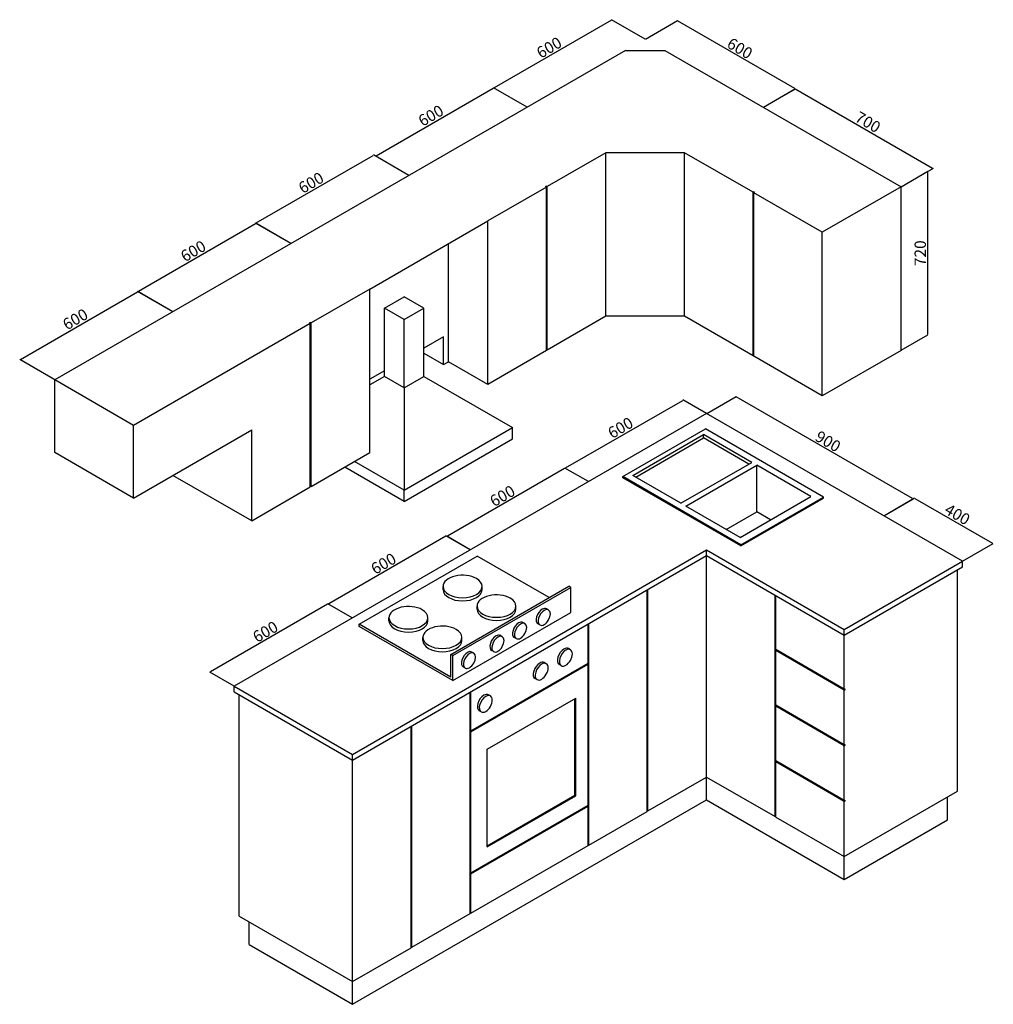
# Model space of a CAD drawing. Units: millimetres. Extents: x 2103 to 6389, y -1168 to 3165.
import ezdxf

# ---------------------------------------------------------------- set-up
doc = ezdxf.new("R2010")
doc.units = ezdxf.units.MM
doc.layers.add('A-ANNO-DIMS', color=2, linetype='Continuous', lineweight=18)
doc.layers.add('A-FURN', color=7, linetype='Continuous', lineweight=25)
doc.styles.get("Standard").update_dxf_attribs({"font": 'arial.ttf'})
doc.dimstyles.new('ISO-25', dxfattribs={"dimtxt": 50, "dimasz": 2.5, "dimexe": 1.25, "dimexo": 0.625, "dimtad": 1, "dimdec": 0, "dimtxsty": 'Standard', "dimcen": 2.5, "dimadec": 0, "dimazin": 0, "dimtfac": 1, "dimtdec": 0, "dimtmove": 0, "dimatfit": 3, "dimfxl": 1, "dimarcsym": 0})

# ---------------------------------------------------------------- blocks, each defined once
blk = doc.blocks.new('*D1')
at = {"layer": 'A-ANNO-DIMS', "color": 0, "lineweight": -2, "transparency": 16777216}
for p, q in [((2106.7, 1670), (2622, 1967.5)), ((2777.4, 1880.3), (2622.9, 1969.5)), ((2257.8, 1580.3), (2103.3, 1669.5))]:
    blk.add_line(p, q, dxfattribs=at)
at = {"layer": 'A-ANNO-DIMS', "color": 0, "transparency": 16777216}
for points in [[(2621.8, 1967.9), (2622.2, 1967.2), (2624.2, 1968.8)], [(2106.5, 1670.4), (2106.9, 1669.7), (2104.6, 1668.8)]]:
    blk.add_solid(points, dxfattribs=at)
at = {"layer": 'Defpoints', "color": 0, "transparency": 16777216}
for p in [(2624.2, 1968.8), (2778, 1879.9), (2258.4, 1579.9)]:
    blk.add_point(p, dxfattribs=at)
at = {"layer": 'A-ANNO-DIMS', "color": 0, "transparency": 16777216, "insert": (2351.3, 1841.4), "char_height": 50, "attachment_point": 5, "rotation": 30}
blk.add_mtext('600', dxfattribs=at)
blk = doc.blocks.new('*D2')
at = {"layer": 'A-ANNO-DIMS', "color": 0, "lineweight": -2, "transparency": 16777216}
for p, q in [((2626, 1970.2), (3141.2, 2267.7)), ((3297, 2180.3), (3142.2, 2269.7)), ((2777.4, 1880.3), (2622.5, 1969.7))]:
    blk.add_line(p, q, dxfattribs=at)
at = {"layer": 'A-ANNO-DIMS', "color": 0, "transparency": 16777216}
for points in [[(3141, 2268.1), (3141.5, 2267.4), (3143.4, 2269)], [(2625.8, 1970.6), (2626.2, 1969.9), (2623.8, 1969)]]:
    blk.add_solid(points, dxfattribs=at)
at = {"layer": 'Defpoints', "color": 0, "transparency": 16777216}
for p in [(3143.4, 2269), (3297.7, 2179.9), (2778, 1879.9)]:
    blk.add_point(p, dxfattribs=at)
at = {"layer": 'A-ANNO-DIMS', "color": 0, "transparency": 16777216, "insert": (2870.5, 2141.6), "char_height": 50, "attachment_point": 5, "rotation": 30}
blk.add_mtext('600', dxfattribs=at)
blk = doc.blocks.new('*D3')
at = {"layer": 'A-ANNO-DIMS', "color": 0, "lineweight": -2, "transparency": 16777216}
for p, q in [((3144.5, 2270.9), (3659.8, 2568.4)), ((3816.6, 2480.3), (3660.7, 2570.4)), ((3297, 2180.3), (3141.1, 2270.4))]:
    blk.add_line(p, q, dxfattribs=at)
at = {"layer": 'A-ANNO-DIMS', "color": 0, "transparency": 16777216}
for points in [[(3659.5, 2568.7), (3660, 2568), (3661.9, 2569.6)], [(3144.3, 2271.2), (3144.7, 2270.5), (3142.3, 2269.6)]]:
    blk.add_solid(points, dxfattribs=at)
at = {"layer": 'Defpoints', "color": 0, "transparency": 16777216}
for p in [(3661.9, 2569.6), (3817.3, 2479.9), (3297.7, 2179.9)]:
    blk.add_point(p, dxfattribs=at)
at = {"layer": 'A-ANNO-DIMS', "color": 0, "transparency": 16777216, "insert": (3389, 2442.3), "char_height": 50, "attachment_point": 5, "rotation": 30}
blk.add_mtext('600', dxfattribs=at)
blk = doc.blocks.new('*D4')
at = {"layer": 'A-ANNO-DIMS', "color": 0, "lineweight": -2, "transparency": 16777216}
for p, q in [((3671.8, 2566.4), (4187.1, 2863.9)), ((4336.3, 2780.3), (4188, 2865.9)), ((3816.6, 2480.3), (3668.4, 2565.9))]:
    blk.add_line(p, q, dxfattribs=at)
at = {"layer": 'A-ANNO-DIMS', "color": 0, "transparency": 16777216}
for points in [[(4186.9, 2864.3), (4187.3, 2863.5), (4189.3, 2865.2)], [(3671.6, 2566.8), (3672.1, 2566), (3669.7, 2565.2)]]:
    blk.add_solid(points, dxfattribs=at)
at = {"layer": 'Defpoints', "color": 0, "transparency": 16777216}
for p in [(4189.3, 2865.2), (4336.9, 2779.9), (3817.3, 2479.9)]:
    blk.add_point(p, dxfattribs=at)
at = {"layer": 'A-ANNO-DIMS', "color": 0, "transparency": 16777216, "insert": (3916.4, 2737.8), "char_height": 50, "attachment_point": 5, "rotation": 30}
blk.add_mtext('600', dxfattribs=at)
blk = doc.blocks.new('*D5')
at = {"layer": 'A-ANNO-DIMS', "color": 0, "lineweight": -2, "transparency": 16777216}
for p, q in [((5983, 2430.3), (6100.8, 2498.4)), ((6099.6, 2495.1), (6099.6, 1780.1)), ((5983, 1710.3), (6100.8, 1778.4))]:
    blk.add_line(p, q, dxfattribs=at)
at = {"layer": 'A-ANNO-DIMS', "color": 0, "transparency": 16777216}
for points in [[(6099.2, 2495.1), (6100, 2495.1), (6099.6, 2497.6)], [(6099.2, 1780.1), (6100, 1780.1), (6099.6, 1777.6)]]:
    blk.add_solid(points, dxfattribs=at)
at = {"layer": 'Defpoints', "color": 0, "transparency": 16777216}
for p in [(5982.3, 2429.9), (6099.6, 1777.6), (5982.3, 1709.9)]:
    blk.add_point(p, dxfattribs=at)
at = {"layer": 'A-ANNO-DIMS', "color": 0, "transparency": 16777216, "insert": (6073.4, 2137.6), "char_height": 50, "attachment_point": 5, "rotation": 90}
blk.add_mtext('720', dxfattribs=at)
blk = doc.blocks.new('*D6')
at = {"layer": 'A-ANNO-DIMS', "color": 0, "lineweight": -2, "transparency": 16777216}
for p, q in [((5376.7, 2780.3), (5518.4, 2862.1)), ((5519.3, 2860.1), (6121.2, 2512.6)), ((5983, 2430.3), (6124.6, 2512.1))]:
    blk.add_line(p, q, dxfattribs=at)
at = {"layer": 'A-ANNO-DIMS', "color": 0, "transparency": 16777216}
for points in [[(5519.5, 2860.5), (5519.1, 2859.7), (5517.1, 2861.4)], [(6121.4, 2513), (6121, 2512.2), (6123.3, 2511.4)]]:
    blk.add_solid(points, dxfattribs=at)
at = {"layer": 'Defpoints', "color": 0, "transparency": 16777216}
for p in [(5376.1, 2779.9), (6123.3, 2511.4), (5982.3, 2429.9)]:
    blk.add_point(p, dxfattribs=at)
at = {"layer": 'A-ANNO-DIMS', "color": 0, "transparency": 16777216, "insert": (5833.3, 2709), "char_height": 50, "attachment_point": 5, "rotation": 330}
blk.add_mtext('700', dxfattribs=at)
blk = doc.blocks.new('*D7')
at = {"layer": 'A-ANNO-DIMS', "color": 0, "lineweight": -2, "transparency": 16777216}
for p, q in [((5906.5, 982.2), (6042.1, 1060.5)), ((6043, 1058.6), (6385.1, 861.1)), ((6252.9, 782.2), (6388.5, 860.5))]:
    blk.add_line(p, q, dxfattribs=at)
at = {"layer": 'A-ANNO-DIMS', "color": 0, "transparency": 16777216}
for points in [[(6043.2, 1058.9), (6042.8, 1058.2), (6040.9, 1059.8)], [(6385.3, 861.4), (6384.9, 860.7), (6387.3, 859.8)]]:
    blk.add_solid(points, dxfattribs=at)
at = {"layer": 'Defpoints', "color": 0, "transparency": 16777216}
for p in [(5905.9, 981.9), (6387.3, 859.8), (6252.3, 781.9)]:
    blk.add_point(p, dxfattribs=at)
at = {"layer": 'A-ANNO-DIMS', "color": 0, "transparency": 16777216, "insert": (6227.1, 982.5), "char_height": 50, "attachment_point": 5, "rotation": 330}
blk.add_mtext('400', dxfattribs=at)
blk = doc.blocks.new('*D8')
at = {"layer": 'A-ANNO-DIMS', "color": 0, "lineweight": -2, "transparency": 16777216}
for p, q in [((5127.1, 1432.2), (5256.3, 1506.8)), ((6032.3, 1057.4), (5257.2, 1504.9)), ((5906.5, 982.2), (6035.7, 1056.8))]:
    blk.add_line(p, q, dxfattribs=at)
at = {"layer": 'A-ANNO-DIMS', "color": 0, "transparency": 16777216}
for points in [[(5257.4, 1505.2), (5257, 1504.5), (5255.1, 1506.1)], [(6032.5, 1057.7), (6032.1, 1057), (6034.5, 1056.1)]]:
    blk.add_solid(points, dxfattribs=at)
at = {"layer": 'Defpoints', "color": 0, "transparency": 16777216}
for p in [(5255.1, 1506.1), (5126.4, 1431.9), (5905.9, 981.9)]:
    blk.add_point(p, dxfattribs=at)
at = {"layer": 'A-ANNO-DIMS', "color": 0, "transparency": 16777216, "insert": (5657.9, 1303.8), "char_height": 50, "attachment_point": 5, "rotation": 330}
blk.add_mtext('900', dxfattribs=at)
blk = doc.blocks.new('*D9')
at = {"layer": 'A-ANNO-DIMS', "color": 0, "lineweight": -2, "transparency": 16777216}
for p, q in [((4506.2, 1192.4), (5021.5, 1489.9)), ((5125.8, 1432.2), (5022.4, 1491.9)), ((4606.2, 1132.2), (4502.8, 1191.9))]:
    blk.add_line(p, q, dxfattribs=at)
at = {"layer": 'A-ANNO-DIMS', "color": 0, "transparency": 16777216}
for points in [[(5021.3, 1490.3), (5021.7, 1489.6), (5023.7, 1491.2)], [(4506, 1192.8), (4506.4, 1192.1), (4504.1, 1191.2)]]:
    blk.add_solid(points, dxfattribs=at)
at = {"layer": 'Defpoints', "color": 0, "transparency": 16777216}
for p in [(5023.7, 1491.2), (5126.4, 1431.9), (4606.8, 1131.9)]:
    blk.add_point(p, dxfattribs=at)
at = {"layer": 'A-ANNO-DIMS', "color": 0, "transparency": 16777216, "insert": (4750.8, 1363.8), "char_height": 50, "attachment_point": 5, "rotation": 30}
blk.add_mtext('600', dxfattribs=at)
blk = doc.blocks.new('*D10')
at = {"layer": 'A-ANNO-DIMS', "color": 0, "lineweight": -2, "transparency": 16777216}
for p, q in [((4501.9, 1189.9), (3986.6, 892.4)), ((4606.2, 1132.2), (4502.8, 1191.9)), ((4086.6, 832.2), (3983.2, 891.9))]:
    blk.add_line(p, q, dxfattribs=at)
at = {"layer": 'A-ANNO-DIMS', "color": 0, "transparency": 16777216}
for points in [[(4501.7, 1190.3), (4502.1, 1189.6), (4504.1, 1191.2)], [(3986.4, 892.8), (3986.8, 892.1), (3984.5, 891.2)]]:
    blk.add_solid(points, dxfattribs=at)
at = {"layer": 'Defpoints', "color": 0, "transparency": 16777216}
for p in [(4606.8, 1131.9), (3984.5, 891.2), (4087.2, 831.9)]:
    blk.add_point(p, dxfattribs=at)
at = {"layer": 'A-ANNO-DIMS', "color": 0, "transparency": 16777216, "insert": (4231.2, 1063.8), "char_height": 50, "attachment_point": 5, "rotation": 30}
blk.add_mtext('600', dxfattribs=at)
blk = doc.blocks.new('*D11')
at = {"layer": 'A-ANNO-DIMS', "color": 0, "lineweight": -2, "transparency": 16777216}
for p, q in [((3978.6, 892), (3463.3, 594.5)), ((4086.6, 832.2), (3979.5, 894)), ((3567, 532.2), (3459.9, 594))]:
    blk.add_line(p, q, dxfattribs=at)
at = {"layer": 'A-ANNO-DIMS', "color": 0, "transparency": 16777216}
for points in [[(3978.4, 892.4), (3978.8, 891.7), (3980.8, 893.3)], [(3463.1, 594.9), (3463.5, 594.2), (3461.2, 593.3)]]:
    blk.add_solid(points, dxfattribs=at)
at = {"layer": 'Defpoints', "color": 0, "transparency": 16777216}
for p in [(4087.2, 831.9), (3461.2, 593.3), (3567.6, 531.9)]:
    blk.add_point(p, dxfattribs=at)
at = {"layer": 'A-ANNO-DIMS', "color": 0, "transparency": 16777216, "insert": (3707.9, 765.9), "char_height": 50, "attachment_point": 5, "rotation": 30}
blk.add_mtext('600', dxfattribs=at)
blk = doc.blocks.new('*D12')
at = {"layer": 'A-ANNO-DIMS', "color": 0, "lineweight": -2, "transparency": 16777216}
for p, q in [((3458.6, 592.3), (2943.3, 294.8)), ((3567, 532.2), (3459.5, 594.3)), ((3047.3, 232.2), (2939.9, 294.3))]:
    blk.add_line(p, q, dxfattribs=at)
at = {"layer": 'A-ANNO-DIMS', "color": 0, "transparency": 16777216}
for points in [[(3458.3, 592.7), (3458.8, 591.9), (3460.7, 593.6)], [(2943.1, 295.2), (2943.5, 294.4), (2941.1, 293.6)]]:
    blk.add_solid(points, dxfattribs=at)
at = {"layer": 'Defpoints', "color": 0, "transparency": 16777216}
for p in [(3567.6, 531.9), (2941.1, 293.6), (3048, 231.9)]:
    blk.add_point(p, dxfattribs=at)
at = {"layer": 'A-ANNO-DIMS', "color": 0, "transparency": 16777216, "insert": (3187.8, 466.2), "char_height": 50, "attachment_point": 5, "rotation": 30}
blk.add_mtext('600', dxfattribs=at)
blk = doc.blocks.new('*D13')
at = {"layer": 'A-ANNO-DIMS', "color": 0, "lineweight": -2, "transparency": 16777216}
for p, q in [((4855.9, 3080.3), (4708.5, 3165.4)), ((4707.6, 3163.4), (4192.3, 2865.9)), ((4336.3, 2780.3), (4188.9, 2865.4))]:
    blk.add_line(p, q, dxfattribs=at)
at = {"layer": 'A-ANNO-DIMS', "color": 0, "transparency": 16777216}
for points in [[(4707.3, 3163.8), (4707.8, 3163.1), (4709.7, 3164.7)], [(4192.1, 2866.3), (4192.5, 2865.6), (4190.1, 2864.7)]]:
    blk.add_solid(points, dxfattribs=at)
at = {"layer": 'Defpoints', "color": 0, "transparency": 16777216}
for p in [(4856.5, 3079.9), (4190.1, 2864.7), (4336.9, 2779.9)]:
    blk.add_point(p, dxfattribs=at)
at = {"layer": 'A-ANNO-DIMS', "color": 0, "transparency": 16777216, "insert": (4436.8, 3037.3), "char_height": 50, "attachment_point": 5, "rotation": 30}
blk.add_mtext('600', dxfattribs=at)
blk = doc.blocks.new('*D14')
at = {"layer": 'A-ANNO-DIMS', "color": 0, "lineweight": -2, "transparency": 16777216}
for p, q in [((4857.1, 3080.3), (4998.2, 3161.8)), ((5514.4, 2862.3), (4999.1, 3159.8)), ((5376.7, 2780.3), (5517.8, 2861.8))]:
    blk.add_line(p, q, dxfattribs=at)
at = {"layer": 'A-ANNO-DIMS', "color": 0, "transparency": 16777216}
for points in [[(4999.3, 3160.2), (4998.9, 3159.4), (4997, 3161)], [(5514.6, 2862.7), (5514.2, 2861.9), (5516.6, 2861)]]:
    blk.add_solid(points, dxfattribs=at)
at = {"layer": 'Defpoints', "color": 0, "transparency": 16777216}
for p in [(4997, 3161), (4856.5, 3079.9), (5376.1, 2779.9)]:
    blk.add_point(p, dxfattribs=at)
at = {"layer": 'A-ANNO-DIMS', "color": 0, "transparency": 16777216, "insert": (5269.8, 3033.7), "char_height": 50, "attachment_point": 5, "rotation": 330}
blk.add_mtext('600', dxfattribs=at)

msp = doc.modelspace()

# ---------------------------------------------------------------- linework, layer by layer
at = {"layer": 'A-FURN'}
for p, q in [((4769.9, 3029.9), (2258.4, 1579.9)), ((4769.9, 3029.9), (4943.1, 3029.9)), ((4943.1, 3029.9), (5982.3, 2429.9)), ((4683.3, 2579.9), (4425.2, 2430.9)), ((4683.3, 1859.9), (4683.3, 2579.9)), ((5029.7, 2579.9), (4683.3, 2579.9)), ((5029.7, 1859.9), (5029.7, 2579.9)), ((5331.1, 2405.9), (5029.7, 2579.9)), ((4421.8, 2428.9), (4163.7, 2279.9)), ((4418.3, 2430.9), (4421.8, 2432.9)), ((4421.8, 2428.9), (4418.3, 2430.9)), ((4421.8, 2428.9), (4421.8, 2432.9)), ((4425.2, 2430.9), (4421.8, 2432.9)), ((4421.8, 1708.9), (4421.8, 2428.9)), ((4425.2, 1710.9), (4425.2, 2430.9)), ((5982.3, 2429.9), (5635.9, 2229.9)), ((5982.3, 1709.9), (5982.3, 2429.9)), ((5331.1, 2405.9), (5334.5, 2407.9)), ((5331.1, 1685.9), (5331.1, 2405.9)), ((5334.5, 2403.9), (5334.5, 2407.9)), ((5338, 2405.9), (5334.5, 2407.9)), ((5334.5, 2403.9), (5338, 2405.9)), ((5334.5, 1683.9), (5334.5, 2403.9)), ((5635.9, 2229.9), (5334.5, 2403.9)), ((3644.1, 1979.9), (4163.7, 2279.9)), ((4163.7, 1559.9), (4163.7, 2279.9)), ((5635.9, 1509.9), (5635.9, 2229.9)), ((3990.5, 1659.9), (3990.5, 2179.9)), ((3644.1, 1979.9), (3386, 1830.9)), ((3644.1, 1259.9), (3644.1, 1979.9)), ((3709, 1895.2), (3795.6, 1945.2)), ((3882.2, 1895.2), (3795.6, 1945.2)), ((3709, 1595.2), (3709, 1895.2)), ((3795.6, 1845.2), (3709, 1895.2)), ((3795.6, 1845.2), (3882.2, 1895.2)), ((3882.2, 1595.2), (3882.2, 1895.2)), ((3382.5, 1828.9), (2604.8, 1379.9)), ((3379.1, 1830.9), (3382.5, 1832.9)), ((3382.5, 1828.9), (3379.1, 1830.9)), ((3386, 1830.9), (3382.5, 1832.9)), ((3382.5, 1828.9), (3382.5, 1832.9)), ((3382.5, 1108.9), (3382.5, 1828.9)), ((3386, 1110.9), (3386, 1830.9)), ((3795.6, 1545.2), (3795.6, 1845.2)), ((4683.3, 1859.9), (4425.2, 1710.9)), ((5029.7, 1859.9), (4683.3, 1859.9)), ((5331.1, 1685.9), (5029.7, 1859.9)), ((3968.8, 1770.2), (3882.2, 1720.2)), ((3968.8, 1647.4), (3968.8, 1770.2)), ((3882.2, 1697.4), (3968.8, 1647.4)), ((4421.8, 1708.9), (4163.7, 1559.9)), ((4425.2, 1710.9), (4421.8, 1712.9)), ((5982.3, 1709.9), (5635.9, 1509.9)), ((3968.8, 1647.4), (3990.5, 1659.9)), ((4163.7, 1559.9), (3990.5, 1659.9)), ((5331.1, 1685.9), (5334.5, 1687.9)), ((5635.9, 1509.9), (5334.5, 1683.9)), ((3709, 1620.2), (3644.1, 1582.7)), ((2604.8, 1379.9), (2258.4, 1579.9)), ((2258.4, 1259.9), (2258.4, 1579.9)), ((3709, 1595.2), (3644.1, 1557.7)), ((3795.6, 1545.2), (3709, 1595.2)), ((3795.6, 1545.2), (3882.2, 1595.2)), ((3882.2, 1595.2), (4271.9, 1370.2)), ((3795.6, 1545.2), (3795.6, 1095.2)), ((5126.4, 1431.9), (3048, 231.9)), ((6252.3, 781.9), (5126.4, 1431.9)), ((2604.8, 1059.9), (2604.8, 1379.9)), ((2604.8, 1059.9), (3124.4, 1359.9)), ((3124.4, 959.9), (3124.4, 1359.9)), ((3795.6, 1095.2), (4271.9, 1370.2)), ((4271.9, 1320.2), (4271.9, 1370.2)), ((4758.4, 1154.4), (5122.1, 1364.4)), ((5641.7, 1064.4), (5122.1, 1364.4)), ((3795.6, 1045.2), (4271.9, 1320.2)), ((4801.7, 1159.4), (5113.4, 1339.4)), ((4814.7, 1151.9), (5113.4, 1324.4)), ((5325.6, 1216.9), (5113.4, 1339.4)), ((5113.4, 1324.4), (5113.4, 1339.4)), ((5312.6, 1209.4), (5113.4, 1324.4)), ((2604.8, 1059.9), (2258.4, 1259.9)), ((3386, 1110.9), (3644.1, 1259.9)), ((3795.6, 1095.2), (3577.2, 1221.3)), ((5013.8, 1036.9), (5325.6, 1216.9)), ((3795.6, 1045.2), (3533.9, 1196.3)), ((5035.5, 1024.4), (5347.3, 1204.4)), ((5585.4, 1066.9), (5347.3, 1204.4)), ((5347.3, 999.4), (5347.3, 1204.4)), ((3124.4, 959.9), (2778, 1159.9)), ((4758.4, 1149.4), (4758.4, 1154.4)), ((5278, 854.4), (4758.4, 1154.4)), ((5278, 849.4), (4758.4, 1149.4)), ((5013.8, 1036.9), (4801.7, 1159.4)), ((3124.4, 959.9), (3382.5, 1108.9)), ((3386, 1110.9), (3382.5, 1112.9)), ((3795.6, 1045.2), (3795.6, 1095.2)), ((5273.7, 886.9), (5585.4, 1066.9)), ((5278, 854.4), (5641.7, 1064.4)), ((5278, 849.4), (5641.7, 1059.4)), ((5641.7, 1059.4), (5641.7, 1064.4)), ((5273.7, 886.9), (5035.5, 1024.4)), ((5213, 921.9), (5347.3, 999.4)), ((5407.9, 964.4), (5347.3, 999.4)), ((3567.6, -68.1), (5126.4, 831.9)), ((5126.4, 806.9), (5126.4, 831.9)), ((5126.4, 831.9), (5732.6, 481.9)), ((5278, 849.4), (5278, 854.4)), ((3567.6, -93.1), (5126.4, 806.9)), ((3597.9, 504.4), (4117.5, 804.4)), ((4433.6, 621.9), (4117.5, 804.4)), ((5126.4, 806.9), (5732.6, 456.9)), ((5126.4, -168.1), (5126.4, 806.9)), ((5732.6, 481.9), (6252.3, 781.9)), ((6252.3, 756.9), (6252.3, 781.9)), ((5732.6, 456.9), (6252.3, 756.9)), ((6230.6, -230.6), (6230.6, 744.4)), ((3966.8, 656.9), (3966.8, 670.9)), ((4000.6, 371.9), (4520.2, 671.9)), ((4009.3, 366.9), (4528.9, 666.9)), ((4138.3, 656.9), (4138.3, 670.9)), ((4528.9, 666.9), (4520.2, 671.9)), ((4528.9, 556.9), (4528.9, 666.9)), ((4864.9, -319.1), (4864.9, 655.9)), ((4868.4, -317.1), (4868.4, 657.9)), ((5427.8, -342.1), (5427.8, 632.9)), ((5431.3, 392.9), (5431.3, 630.9)), ((4116.2, 570.6), (4116.2, 584.6)), ((4287.7, 570.6), (4287.7, 584.6)), ((4430.9, 567.2), (4422.3, 572.2)), ((3728.7, 519.4), (3728.7, 533.4)), ((3900.1, 519.4), (3900.1, 533.4)), ((4009.3, 256.9), (4528.9, 556.9)), ((4000.6, 271.9), (3597.9, 504.4)), ((3597.9, 494.4), (3597.9, 504.4)), ((4009.3, 256.9), (3597.9, 494.4)), ((4327, 507.2), (4318.4, 512.2)), ((4393, 501.5), (4384.3, 506.5)), ((4605.1, 332.9), (4605.1, 505.9)), ((4608.5, -467.1), (4608.5, 507.9)), ((5732.6, 456.9), (5732.6, 481.9)), ((3878.1, 433.1), (3878.1, 447.1)), ((4049.5, 433.1), (4049.5, 447.1)), ((4227.4, 449.7), (4218.8, 454.7)), ((4289.1, 441.5), (4280.4, 446.5)), ((5732.6, 218.9), (5732.6, 456.9)), ((4527.4, 392.4), (4518.8, 397.4)), ((5732.6, 218.9), (5431.3, 392.9)), ((5431.3, 388.9), (5431.3, 392.9)), ((5431.3, 388.9), (5434.7, 390.9)), ((4009.3, 366.9), (4000.6, 371.9)), ((4000.6, 271.9), (4000.6, 371.9)), ((4009.3, 256.9), (4009.3, 366.9)), ((4101.9, 377.2), (4093.2, 382.2)), ((4189.5, 384), (4180.8, 389)), ((5732.6, 214.9), (5431.3, 388.9)), ((5431.3, 147.9), (5431.3, 388.9)), ((4063.9, 311.5), (4055.2, 316.5)), ((4088.9, 34.9), (4605.1, 332.9)), ((4088.9, 30.9), (4605.1, 328.9)), ((4420.9, 330.9), (4412.2, 335.9)), ((4487, 322.4), (4478.4, 327.4)), ((4601.6, 330.9), (4605.1, 328.9)), ((4605.1, 328.9), (4605.1, 332.9)), ((4605.1, -292.1), (4605.1, 328.9)), ((4380.5, 260.9), (4371.8, 265.9)), ((3048, 206.9), (3048, 231.9)), ((3048, 231.9), (3567.6, -68.1)), ((5732.6, 218.9), (5736.1, 220.9)), ((5736.1, 216.9), (5732.6, 218.9)), ((5732.6, 214.9), (5736.1, 216.9)), ((5736.1, 216.9), (5736.1, 220.9)), ((3048, 206.9), (3567.6, -93.1)), ((3069.6, -780.6), (3069.6, 194.4)), ((4085.5, -769.1), (4085.5, 205.9)), ((4088.9, 34.9), (4088.9, 207.9)), ((4160.8, -45.6), (4550.5, 179.4)), ((4175, 188.9), (4166.3, 193.9)), ((4546.2, -248.1), (4546.2, 176.9)), ((4550.5, -250.6), (4550.5, 179.4)), ((5732.6, -26.1), (5732.6, 214.9)), ((5431.3, 143.9), (5431.3, 147.9)), ((5732.6, -26.1), (5431.3, 147.9)), ((5431.3, 143.9), (5434.7, 145.9)), ((5732.6, -30.1), (5431.3, 143.9)), ((5431.3, -97.1), (5431.3, 143.9)), ((4134.5, 118.9), (4125.9, 123.9)), ((3825.7, -919.1), (3825.7, 55.9)), ((3829.1, -917.1), (3829.1, 57.9)), ((4085.5, 36.9), (4088.9, 34.9)), ((4085.5, 32.9), (4088.9, 34.9)), ((4085.5, 32.9), (4088.9, 30.9)), ((4088.9, -590.1), (4088.9, 30.9)), ((5732.6, -26.1), (5736.1, -24.1)), ((5736.1, -28.1), (5732.6, -26.1)), ((5732.6, -30.1), (5736.1, -28.1)), ((5732.6, -271.1), (5732.6, -30.1)), ((5736.1, -28.1), (5736.1, -24.1)), ((3567.6, -93.1), (3567.6, -68.1)), ((4160.8, -475.6), (4160.8, -45.6)), ((3567.6, -1068.1), (3567.6, -93.1)), ((5431.3, -101.1), (5431.3, -97.1)), ((5732.6, -271.1), (5431.3, -97.1)), ((5431.3, -101.1), (5434.7, -99.1)), ((5732.6, -275.1), (5431.3, -101.1)), ((5431.3, -344.1), (5431.3, -101.1)), ((4868.4, -317.1), (5126.4, -168.1)), ((5126.4, -268.1), (5126.4, -168.1)), ((5126.4, -168.1), (5427.8, -342.1)), ((4160.8, -470.6), (4546.2, -248.1)), ((4160.8, -475.6), (4550.5, -250.6)), ((4550.5, -250.6), (4546.2, -248.1)), ((5732.6, -518.1), (6230.6, -230.6)), ((6187.3, -355.6), (6187.3, -255.6)), ((3567.6, -1168.1), (5126.4, -268.1)), ((4088.9, -590.1), (4605.1, -292.1)), ((4088.9, -594.1), (4605.1, -296.1)), ((4601.6, -294.1), (4605.1, -296.1)), ((4605.1, -296.1), (4605.1, -292.1)), ((4605.1, -469.1), (4605.1, -296.1)), ((5126.4, -268.1), (5732.6, -618.1)), ((5732.6, -271.1), (5736.1, -269.1)), ((5736.1, -273.1), (5732.6, -271.1)), ((5732.6, -275.1), (5736.1, -273.1)), ((5732.6, -518.1), (5732.6, -275.1)), ((5736.1, -273.1), (5736.1, -269.1)), ((4608.5, -467.1), (4864.9, -319.1)), ((4868.4, -317.1), (4864.9, -315.1)), ((5427.8, -342.1), (5431.3, -340.1)), ((5431.3, -344.1), (5732.6, -518.1)), ((5732.6, -618.1), (6187.3, -355.6)), ((4088.9, -767.1), (4605.1, -469.1)), ((4608.5, -467.1), (4605.1, -465.1)), ((5732.6, -618.1), (5732.6, -518.1)), ((4085.5, -588.1), (4088.9, -590.1)), ((4085.5, -592.1), (4088.9, -590.1)), ((4085.5, -592.1), (4088.9, -594.1)), ((4088.9, -767.1), (4088.9, -594.1)), ((3829.1, -917.1), (4085.5, -769.1)), ((4088.9, -767.1), (4085.5, -765.1)), ((3069.6, -780.6), (3567.6, -1068.1)), ((3112.9, -905.6), (3112.9, -805.6)), ((3112.9, -905.6), (3567.6, -1168.1)), ((3567.6, -1068.1), (3825.7, -919.1)), ((3829.1, -917.1), (3825.7, -915.1)), ((3567.6, -1168.1), (3567.6, -1068.1))]:
    msp.add_line(p, q, dxfattribs=at)
for centre, major_axis, start_param, end_param in [((4052.6, 670.9), (85.7, 0), 0.785398, 3.141593), ((4052.6, 670.9), (85.7, 0), 0, 0.785398), ((4052.6, 670.9), (85.7, 0), 3.141593, 6.283185), ((4052.6, 656.9), (85.7, 0), 3.141593, 6.283185), ((4201.9, 584.6), (85.7, 0), 0.785398, 3.141593), ((4201.9, 584.6), (85.7, 0), 0, 0.785398), ((3814.4, 533.4), (85.7, 0), 0.785398, 3.141593), ((3814.4, 533.4), (85.7, 0), 0, 0.785398), ((4201.9, 584.6), (85.7, 0), 3.141593, 6.283185), ((4201.9, 570.6), (85.7, 0), 3.141593, 6.283185), ((4403.3, 539.4), (19, 32.9), 0.785398, 3.141593), ((4412, 534.4), (19, 32.9), 0.785398, 3.141593), ((4412, 534.4), (19, 32.9), 3.141593, 6.283185), ((4403.3, 539.4), (19, 32.9), 0, 0.785398), ((4412, 534.4), (19, 32.9), 0, 0.785398), ((3814.4, 533.4), (85.7, 0), 3.141593, 6.283185), ((3814.4, 519.4), (85.7, 0), 3.141593, 6.283185), ((3963.8, 447.1), (85.7, 0), 0.785398, 3.141593), ((3963.8, 447.1), (85.7, 0), 0, 0.785398), ((4299.4, 479.4), (19, 32.9), 0.785398, 3.141593), ((4308, 474.4), (19, 32.9), 0.785398, 3.141593), ((4308, 474.4), (19, 32.9), 3.141593, 6.283185), ((4299.4, 479.4), (19, 32.9), 0, 0.785398), ((4308, 474.4), (19, 32.9), 0, 0.785398), ((3963.8, 447.1), (85.7, 0), 3.141593, 6.283185), ((4199.8, 421.9), (19, 32.9), 0.785398, 3.141593), ((4208.4, 416.9), (19, 32.9), 0.785398, 3.141593), ((4208.4, 416.9), (19, 32.9), 3.141593, 6.283185), ((4199.8, 421.9), (19, 32.9), 0, 0.785398), ((4208.4, 416.9), (19, 32.9), 0, 0.785398), ((3963.8, 433.1), (85.7, 0), 3.141593, 6.283185), ((4498.6, 362.4), (20.2, 35), 0.785398, 3.141593), ((4507.2, 357.4), (20.2, 35), 0.785398, 3.141593), ((4507.2, 357.4), (20.2, 35), 3.141593, 6.283185), ((4498.6, 362.4), (20.2, 35), 0, 0.785398), ((4507.2, 357.4), (20.2, 35), 0, 0.785398), ((4074.2, 349.4), (19, 32.9), 0.785398, 3.141593), ((4082.9, 344.4), (19, 32.9), 0.785398, 3.141593), ((4082.9, 344.4), (19, 32.9), 3.141593, 6.283185), ((4074.2, 349.4), (19, 32.9), 0, 0.785398), ((4082.9, 344.4), (19, 32.9), 0, 0.785398), ((4392, 300.9), (20.2, 35), 0.785398, 3.141593), ((4400.7, 295.9), (20.2, 35), 0.785398, 3.141593), ((4400.7, 295.9), (20.2, 35), 3.141593, 6.283185), ((4392, 300.9), (20.2, 35), 0, 0.785398), ((4400.7, 295.9), (20.2, 35), 0, 0.785398), ((4146.1, 158.9), (20.2, 35), 0.785398, 3.141593), ((4154.7, 153.9), (20.2, 35), 0.785398, 3.141593), ((4154.7, 153.9), (20.2, 35), 3.141593, 6.283185), ((4146.1, 158.9), (20.2, 35), 0, 0.785398), ((4154.7, 153.9), (20.2, 35), 0, 0.785398)]:
    msp.add_ellipse(centre, major_axis=major_axis, ratio=0.57735, start_param=start_param, end_param=end_param, dxfattribs=at)

# ---------------------------------------------------------------- dimensions: what is measured, and where the dimension line sits
at = {"layer": 'A-ANNO-DIMS'}
for p1, p2, distance, picture, middle in [((4856.5, 3079.9), (4336.9, 2779.9), -146.8, '*D13', (4436.8, 3037.3)), ((5376.1, 2779.9), (4856.5, 3079.9), -140.5, '*D14', (5269.8, 3033.7)), ((3817.3, 2479.9), (4336.9, 2779.9), 147.6, '*D4', (3916.4, 2737.8)), ((5376.1, 2779.9), (5982.3, 2429.9), 141, '*D6', (5833.3, 2709)), ((3297.7, 2179.9), (3817.3, 2479.9), 155.3, '*D3', (3389, 2442.3)), ((5982.3, 2429.9), (5982.3, 1709.9), 117.3, '*D5', (6073.4, 2137.6)), ((2778, 1879.9), (3297.7, 2179.9), 154.2, '*D2', (2870.5, 2141.6)), ((2258.4, 1579.9), (2778, 1879.9), 153.9, '*D1', (2351.3, 1841.4)), ((5905.9, 981.9), (5126.4, 1431.9), -128.6, '*D8', (5657.9, 1303.8)), ((4606.8, 1131.9), (4087.2, 831.9), -102.7, '*D10', (4231.2, 1063.8)), ((5905.9, 981.9), (6252.3, 781.9), 135, '*D7', (6227.1, 982.5)), ((4087.2, 831.9), (3567.6, 531.9), -106.4, '*D11', (3707.9, 765.9)), ((3567.6, 531.9), (3048, 231.9), -106.9, '*D12', (3187.8, 466.2))]:
    dim = msp.add_aligned_dim(p1=p1, p2=p2, distance=distance, dimstyle='ISO-25', override={"dimclrd": 0, "dimclre": 0, "dimclrt": 0}, dxfattribs=at)
    dim.commit()
    dim.dimension.update_dxf_attribs({"geometry": picture, "text_midpoint": middle})
dim = msp.add_linear_dim(base=(5023.7, 1491.2), p1=(4606.8, 1131.9), p2=(5126.4, 1431.9), angle=30, dimstyle='ISO-25', override={"dimclrd": 0, "dimclre": 0, "dimclrt": 0}, dxfattribs=at)
dim.commit()
dim.dimension.update_dxf_attribs({"geometry": '*D9', "text_midpoint": (4763.9, 1341.2), "dimtype": 161})

doc.saveas('drawing.dxf')
